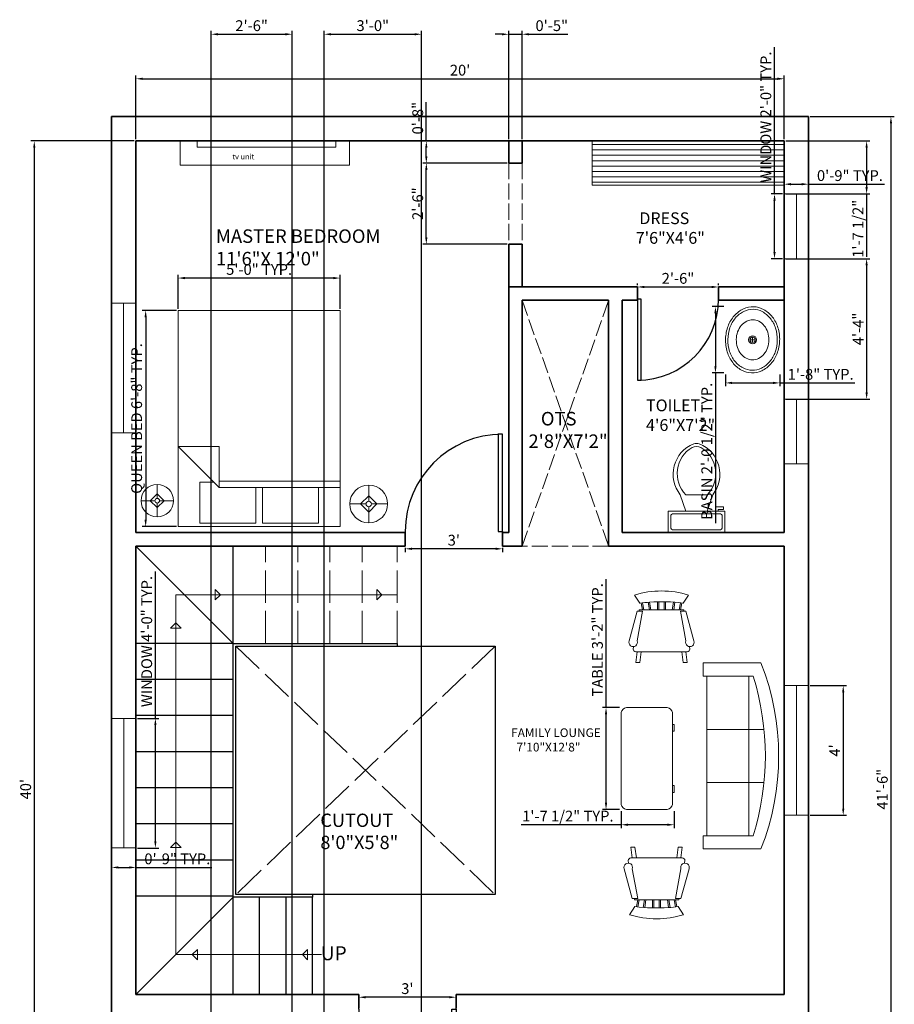
# Model space of a CAD drawing. Units: inches. Extents: x 2170 to 3011, y 1733 to 2338.
# Tile 5 of 5: x 2677 to 3000, y 1974 to 2338. Entities that reach past the tile are written whole.
import ezdxf

# ---------------------------------------------------------------- set-up
doc = ezdxf.new("R2010")
doc.units = ezdxf.units.IN
doc.linetypes.add('ACAD_ISO02W100', pattern=[15, 12, -3])
for name, color, linetype, lineweight in [('A-ANNO-SYMB', 2, 'Continuous', 13), ('A-AREA-IDEN', 4, 'Continuous', 18), ('A-FLOR-CASE', 20, 'Continuous', 20), ('A-FLOR-CASE-PATT', 252, 'Continuous', 13), ('A-FLOR-FIXT', 20, 'Continuous', 18), ('A-FLOR-OPEN', 7, 'Continuous', 25), ('A-FLOR-OPEN-HIDN', 7, 'ACAD_ISO02W100', 13), ('A-FLOR-STRS-OVHD', 150, 'ACAD_ISO02W100', 18), ('A-WALL', 7, 'Continuous', 35), ('A-WALL-OVHD', 7, 'ACAD_ISO02W100', 18), ('dim', 11, 'Continuous', 18), ('door', 6, 'Continuous', 25), ('furnitures', 20, 'Continuous', 18), ('stairs', 150, 'Continuous', 25), ('text', 4, 'Continuous', 18), ('window', 3, 'Continuous', 20)]:
    doc.layers.add(name, color=color, linetype=linetype, lineweight=lineweight)
doc.styles.get("Standard").update_dxf_attribs({"font": 'arial.ttf'})
doc.dimstyles.new('ISO-25', dxfattribs={"dimtxt": 4, "dimasz": 2.5, "dimexe": 1.25, "dimexo": 0.625, "dimtad": 1, "dimlunit": 3, "dimtxsty": 'Standard', "dimcen": 2.5, "dimadec": 0, "dimazin": 0, "dimtfac": 1, "dimtmove": 0, "dimatfit": 3, "dimfxl": 1, "dimarcsym": 0})

# ---------------------------------------------------------------- blocks, each defined once
blk = doc.blocks.new('*U3')
for p, q in [((0, 0), (0, -6)), ((-40, 0), (-40, -6))]:
    blk.add_line(p, q)
blk.add_lwpolyline([(0, 0), (0, 40), (-1.75, 40), (-1.75, 0)], close=True)
blk.add_arc((0, 0), 40, 90, 180)
blk = doc.blocks.new('Toilet - top')
for p, q in [((9.5, -6), (9.5, -2)), ((-10, -8.5), (-8, -8.5)), ((-10, -9.5), (-10, -8.5)), ((-7, -9.5), (-10, -9.5)), ((-8, -8.5), (-8, -8)), ((-7, -8), (-7, -9.5)), ((-4, -8), (-6, -14)), ((4, -8), (6, -14)), ((4, -14), (-4, -14))]:
    blk.add_line(p, q)
blk.add_lwpolyline([(10.5, -8), (10.5, 0), (-10.5, 0), (-10.5, -8)], close=True)
for points in [[(-9.5, -2), (-9.5, -6)], [(8.5, -1), (-8.5, -1)], [(-8.5, -7), (8.5, -7)]]:
    blk.add_lwpolyline(points)
for centre, radius, start, end in [((-8.62, -1.88), 0.884, 81.8699, 188.1301), ((8.62, -1.88), 0.884, 351.8699, 98.1301), ((-8.62, -6.12), 0.884, 171.8699, 278.1301), ((8.62, -6.12), 0.884, 261.8699, 8.1301), ((3.52, -21.58), 12.17, 141.4691, 247.9714), ((4.2, -21.82), 11.33, 136.3677, 238.9468), ((-3.52, -21.58), 12.17, 292.0284, 38.5307), ((-4.2, -21.82), 11.33, 301.053, 43.6321), ((0, -27.88), 4, 245.7318, 294.2682), ((0, -29), 4, 254.8605, 285.1395)]:
    blk.add_arc(centre, radius, start, end)
blk = doc.blocks.new('Bed - Queen')
for p, q in [((0, -80.00003), (0, 0)), ((0, 0), (59.99999, 0)), ((59.99999, 0), (59.99999, -80.00003)), ((7.99999, -1.2), (28.79998, -1.2)), ((7.99999, -14.4), (7.99999, -1.2)), ((28.79998, -1.2), (28.79998, -14.4)), ((31.19999, -1.2), (51.99999, -1.2)), ((31.19999, -14.4), (31.19999, -1.2)), ((51.99999, -1.2), (51.99999, -16.4)), ((0, -14.4), (44.8, -14.4)), ((59.99999, -29.6), (44.8, -14.4)), ((44.8, -14.4), (44.8, -29.6)), ((44.8, -16.8), (0, -16.8)), ((51.99999, -16.4), (46.79936, -16.4)), ((44.8, -29.6), (59.99999, -29.6)), ((59.99999, -80.00003), (0, -80.00003))]:
    blk.add_line(p, q)
blk = doc.blocks.new('Desk - 30 x 60 in.')
for p, q in [((-26.999995, 0), (26.999995, 0)), ((-29.999995, -27), (-29.999995, -3)), ((29.999995, -3), (29.999995, -27)), ((26.999995, -30), (-26.999995, -30)), ((-20.000005, -30), (-20.000005, -31)), ((-20.000005, -31), (-16.000005, -31)), ((-16.000005, -31), (-16.000005, -30)), ((15.999995, -31), (15.999995, -30)), ((19.999995, -31), (15.999995, -31)), ((19.999995, -30), (19.999995, -31))]:
    blk.add_line(p, q)
for centre, start, end in [((-26.499995, -3.5), 98.1301, 171.8699), ((26.499995, -3.5), 8.130102, 81.8699), ((-26.499995, -26.5), 188.1301, 261.8699), ((26.499995, -26.5), 278.1301, 351.8699)]:
    blk.add_arc(centre, 3.535534, start, end)
blk = doc.blocks.new('Sofa - Roundback 7 ft.')
for p, q in [((-12.00002, -32.4421), (-12.00003, -6.5971)), ((11.99997, -32.4421), (11.99998, -6.5971)), ((-36.000027, -34), (-36.000027, -11.4696)), ((35.99998, -34), (35.99998, -11.4696)), ((-35.999844, -13.3819), (35.9998, -13.3819)), ((-36.000027, -32.4421), (35.99998, -32.4421))]:
    blk.add_line(p, q)
for points in [[(-36.000027, -34), (-42.000027, -34), (-42.000027, -8)], [(41.99998, -8), (41.99998, -34), (35.99998, -34)]]:
    blk.add_lwpolyline(points)
for centre, radius, start, end in [((0, -114.25), 114.25, 68.43141, 111.5686), ((-0.00001, -127.1968), 121.1968, 72.72033, 107.2797)]:
    blk.add_arc(centre, radius, start, end)
blk = doc.blocks.new('Lamp - Table')
for p, q in [((0, 7), (0, 1)), ((-1, 0), (-7, 0)), ((0, 3), (-3, 0)), ((-3, 0), (0, -3)), ((3, 0), (0, 3)), ((0, -3), (3, 0)), ((1, 0), (7, 0)), ((0, -1), (0, -7))]:
    blk.add_line(p, q)
for radius in [7, 1]:
    blk.add_circle((0, 0), radius)
blk = doc.blocks.new('Sink - Oval top')
for p, q in [((-1, 0), (1, 0)), ((0, 1), (0, -1))]:
    blk.add_line(p, q)
for points in [[(-12.23, 0.39, 0.117634), (-11.46, -3.36, 0.104469), (-8.88, -6.8, 0.090016), (-5.08, -9.07, 0.08192), (-0.32, -10.02, 0.08192), (4.49, -9.38, 0.090016), (8.42, -7.36, 0.104469), (11.22, -4.09, 0.117634), (12.23, -0.39, 0.117634), (11.46, 3.36, 0.104469), (8.88, 6.8, 0.090016), (5.08, 9.07, 0.08192), (0.32, 10.02, 0.08192), (-4.49, 9.38, 0.090016), (-8.42, 7.36, 0.104469), (-11.22, 4.09, 0.117634)], [(-11.29, 0.16, 0.118622), (-10.52, -3.25, 0.104678), (-8.07, -6.36, 0.089562), (-4.54, -8.37, 0.081185), (-0.13, -9.15, 0.081185), (4.3, -8.49, 0.089562), (7.89, -6.58, 0.104678), (10.42, -3.55, 0.118622), (11.29, -0.16, 0.118622), (10.52, 3.25, 0.104678), (8.07, 6.36, 0.089562), (4.54, 8.37, 0.081185), (0.13, 9.15, 0.081185), (-4.3, 8.49, 0.089562), (-7.89, 6.58, 0.104678), (-10.42, 3.55, 0.118622)], [(-7.42, 0.08, 0.118283), (-6.91, -2.17, 0.104607), (-5.29, -4.21, 0.089718), (-2.97, -5.53, 0.081436), (-0.07, -6.04, 0.081436), (2.84, -5.59, 0.089718), (5.2, -4.33, 0.104607), (6.86, -2.32, 0.118283), (7.42, -0.08, 0.118283), (6.91, 2.17, 0.104607), (5.29, 4.21, 0.089718), (2.97, 5.53, 0.081436), (0.07, 6.04, 0.081436), (-2.84, 5.59, 0.089718), (-5.2, 4.33, 0.104607), (-6.86, 2.32, 0.118283)]]:
    blk.add_lwpolyline(points, format="xyb", close=True)
for radius in [1.5, 1]:
    blk.add_circle((0, 0), radius)
blk = doc.blocks.new('Chair - Rocking')
for p, q in [((-8, -4.5), (-10, -1.5)), ((8, -4.5), (10, -1.5)), ((-8.23428, -6.99939), (-8.3093, -7.47958)), ((-8.23041, -7), (8.23915, -7)), ((-7.5, -4.5), (-7, -7)), ((-6.5, -7), (-7.02225, -4.43)), ((-4.5, -7), (-4.96674, -4.19951)), ((-4, -7), (-4.40532, -4.16272)), ((-1.5, -4.05012), (-1.5, -7)), ((-1, -7), (-1, -4.05012)), ((1, -7), (1, -4.04655)), ((1.5, -4.05012), (1.5, -7)), ((4, -7), (4.40187, -4.18694)), ((4.5, -7), (4.96761, -4.19437)), ((6.5, -7), (7, -4.4057)), ((7.5, -4.5), (7, -7)), ((8.31071, -7.48854), (8.23449, -7.00073)), ((-9, -7.5), (-12, -18.49999)), ((-7, -7.5), (-9, -7.5)), ((-9, -18.49999), (-7, -7.5)), ((7, -7.5), (9, -7.5)), ((9, -18.49999), (7, -7.5)), ((9, -7.5), (12, -18.49999)), ((-10.36644, -20.64523), (-10.5, -21.49999)), ((10.5, -21.49999), (10.3575, -20.58798)), ((-9, -22.49999), (-9.5, -26.49999)), ((0, -22.49999), (-9.5, -22.49999)), ((-8, -26.49999), (-7.5, -22.49999)), ((0, -22.49999), (9.5, -22.49999)), ((8, -26.49999), (7.5, -22.49999)), ((9, -22.49999), (9.5, -26.49999)), ((-9.5, -26.49999), (-8, -26.49999)), ((9.5, -26.49999), (8, -26.49999))]:
    blk.add_line(p, q)
for centre, radius, start, end in [((0, -34.08333), 34.08333, 72.93847, 107.0615), ((0, -68.25004), 64.25, 93.92211, 97.15267), ((0, -68.25004), 64.25, 82.84733, 93.92211), ((-10.5, -18.99999), 1.58114, 161.5651, 18.43495), ((-9.5, -21.49999), 1, 180, 270), ((10.5, -18.99999), 1.58114, 161.5651, 18.43495), ((9.5, -21.49999), 1, 270, 0)]:
    blk.add_arc(centre, radius, start, end)
blk = doc.blocks.new('*D35')
at = {"layer": 'Defpoints', "color": 0, "transparency": 16777216}
for p in [(2959.6, 2316.33), (2719.6, 2293.31), (2959.6, 2293.31)]:
    blk.add_point(p, dxfattribs=at)
at = {"layer": 'dim', "color": 0, "lineweight": -2, "transparency": 16777216}
for p, q in [((2719.6, 2293.93), (2719.6, 2317.58)), ((2722.1, 2316.33), (2957.1, 2316.33)), ((2959.6, 2293.93), (2959.6, 2317.58))]:
    blk.add_line(p, q, dxfattribs=at)
at = {"layer": 'dim', "color": 0, "transparency": 16777216}
for points in [[(2722.1, 2316.74), (2722.1, 2315.91), (2719.6, 2316.33)], [(2957.1, 2316.74), (2957.1, 2315.91), (2959.6, 2316.33)]]:
    blk.add_solid(points, dxfattribs=at)
at = {"layer": 'dim', "color": 0, "transparency": 16777216, "insert": (2839.6, 2318.99), "char_height": 4, "attachment_point": 5}
blk.add_mtext("20'", dxfattribs=at)
blk = doc.blocks.new('*D36')
at = {"layer": 'Defpoints', "color": 0, "transparency": 16777216}
for p in [(2719.6, 2293.31), (2681.96, 1813.31), (2719.6, 1813.31)]:
    blk.add_point(p, dxfattribs=at)
at = {"layer": 'dim', "color": 0, "lineweight": -2, "transparency": 16777216}
for p, q in [((2718.97, 2293.31), (2680.71, 2293.31)), ((2681.96, 2290.81), (2681.96, 1815.81)), ((2718.97, 1813.31), (2680.71, 1813.31))]:
    blk.add_line(p, q, dxfattribs=at)
at = {"layer": 'dim', "color": 0, "transparency": 16777216}
for points in [[(2681.54, 2290.81), (2682.37, 2290.81), (2681.96, 2293.31)], [(2681.54, 1815.81), (2682.37, 1815.81), (2681.96, 1813.31)]]:
    blk.add_solid(points, dxfattribs=at)
at = {"layer": 'dim', "color": 0, "transparency": 16777216, "insert": (2679.29, 2053.31), "char_height": 4, "attachment_point": 5, "rotation": 90}
blk.add_mtext("40'", dxfattribs=at)
blk = doc.blocks.new('*D33')
at = {"layer": 'Defpoints', "color": 0, "transparency": 16777216}
for p in [(2819.27, 2143.31), (2819.27, 2142.31), (2855.27, 2143.31)]:
    blk.add_point(p, dxfattribs=at)
at = {"layer": 'dim', "color": 0, "lineweight": -2, "transparency": 16777216}
for p, q in [((2819.27, 2142.68), (2819.27, 2141.06)), ((2852.77, 2142.31), (2821.77, 2142.31)), ((2855.27, 2142.68), (2855.27, 2141.06))]:
    blk.add_line(p, q, dxfattribs=at)
at = {"layer": 'dim', "color": 0, "transparency": 16777216}
for points in [[(2821.77, 2142.73), (2821.77, 2141.9), (2819.27, 2142.31)], [(2852.77, 2142.73), (2852.77, 2141.9), (2855.27, 2142.31)]]:
    blk.add_solid(points, dxfattribs=at)
at = {"layer": 'dim', "color": 0, "transparency": 16777216, "insert": (2837.27, 2144.98), "char_height": 4, "attachment_point": 5}
blk.add_mtext("3'", dxfattribs=at)
blk = doc.blocks.new('*D34')
at = {"layer": 'Defpoints', "color": 0, "transparency": 16777216}
for p in [(2968.6, 2091.66), (2968.6, 2043.66), (2981.44, 2043.66)]:
    blk.add_point(p, dxfattribs=at)
at = {"layer": 'dim', "color": 0, "lineweight": -2, "transparency": 16777216}
for p, q in [((2969.22, 2091.66), (2982.69, 2091.66)), ((2981.44, 2089.16), (2981.44, 2046.16)), ((2969.22, 2043.66), (2982.69, 2043.66))]:
    blk.add_line(p, q, dxfattribs=at)
at = {"layer": 'dim', "color": 0, "transparency": 16777216}
for points in [[(2981.03, 2089.16), (2981.86, 2089.16), (2981.44, 2091.66)], [(2981.03, 2046.16), (2981.86, 2046.16), (2981.44, 2043.66)]]:
    blk.add_solid(points, dxfattribs=at)
at = {"layer": 'dim', "color": 0, "transparency": 16777216, "insert": (2978.82, 2067.66), "char_height": 4, "attachment_point": 5, "rotation": 90}
blk.add_mtext("4'", dxfattribs=at)
blk = doc.blocks.new('*U37')
for p, q in [((-40, 0), (-40, 6)), ((0, 0), (0, 6))]:
    blk.add_line(p, q)
blk.add_lwpolyline([(0, 0), (0, -40), (-1.75, -40), (-1.75, 0)], close=True)
blk.add_arc((0, 0), 40, 180, 270)
blk = doc.blocks.new('*D41')
at = {"layer": 'Defpoints', "color": 0, "transparency": 16777216}
for p in [(2802.09, 1977.31), (2802.09, 1976.29), (2838.09, 1977.31)]:
    blk.add_point(p, dxfattribs=at)
at = {"layer": 'dim', "color": 0, "lineweight": -2, "transparency": 16777216}
for p, q in [((2802.09, 1976.68), (2802.09, 1975.04)), ((2835.59, 1976.29), (2804.59, 1976.29)), ((2838.09, 1976.68), (2838.09, 1975.04))]:
    blk.add_line(p, q, dxfattribs=at)
at = {"layer": 'dim', "color": 0, "transparency": 16777216}
for points in [[(2804.59, 1976.71), (2804.59, 1975.88), (2802.09, 1976.29)], [(2835.59, 1976.71), (2835.59, 1975.88), (2838.09, 1976.29)]]:
    blk.add_solid(points, dxfattribs=at)
at = {"layer": 'dim', "color": 0, "transparency": 16777216, "insert": (2820.09, 1978.96), "char_height": 4, "attachment_point": 5}
blk.add_mtext("3'", dxfattribs=at)
blk = doc.blocks.new('*D42')
at = {"layer": 'Defpoints', "color": 0, "transparency": 16777216}
for p in [(2905.27, 2239.26), (2935.27, 2239.26), (2935.27, 2239.26)]:
    blk.add_point(p, dxfattribs=at)
at = {"layer": 'dim', "color": 0, "lineweight": -2, "transparency": 16777216}
for p, q in [((2905.27, 2239.88), (2905.27, 2240.51)), ((2907.77, 2239.26), (2932.77, 2239.26)), ((2935.27, 2239.88), (2935.27, 2240.51))]:
    blk.add_line(p, q, dxfattribs=at)
at = {"layer": 'dim', "color": 0, "transparency": 16777216}
for points in [[(2907.77, 2239.67), (2907.77, 2238.84), (2905.27, 2239.26)], [(2932.77, 2239.67), (2932.77, 2238.84), (2935.27, 2239.26)]]:
    blk.add_solid(points, dxfattribs=at)
at = {"layer": 'dim', "color": 0, "transparency": 16777216, "insert": (2920.27, 2241.92), "char_height": 4, "attachment_point": 5}
blk.add_mtext('2\'-6"', dxfattribs=at)
blk = doc.blocks.new('WINDOW-48x9')
blk.add_line((4.5, 48), (4.5, 0))
blk.add_lwpolyline([(0, 48), (9, 48), (9, 0), (0, 0)], close=True)
blk = doc.blocks.new('WINDOW-24x9')
blk.add_line((4.5, 24), (4.5, 0))
blk.add_lwpolyline([(0, 24), (9, 24), (9, 0), (0, 0)], close=True)
blk = doc.blocks.new('STAIR-UP-PATH')
for p, q in [((1.94, 1.94), (1.94, 135.18)), ((1.94, 135.18), (83.94, 135.18)), ((16.56, 133.24), (16.56, 137.12)), ((16.56, 137.12), (18.45, 135.18)), ((16.56, 133.24), (18.45, 135.18)), ((76.31, 133.24), (76.31, 137.12)), ((76.31, 137.12), (78.21, 135.18)), ((76.31, 133.24), (78.21, 135.18)), ((0, 122.86), (1.94, 124.75)), ((3.88, 122.86), (1.94, 124.75)), ((3.88, 122.86), (0, 122.86)), ((0, 41.63), (1.94, 43.52)), ((3.88, 41.63), (0, 41.63)), ((3.88, 41.63), (1.94, 43.52)), ((9.93, 3.88), (8.04, 1.94)), ((9.93, 3.88), (9.93, 0)), ((50.68, 3.88), (48.79, 1.94)), ((50.68, 3.88), (50.68, 0)), ((55.9, 1.94), (1.94, 1.94)), ((9.93, 0), (8.04, 1.94)), ((50.68, 0), (48.79, 1.94))]:
    blk.add_line(p, q)
blk = doc.blocks.new('*D56')
at = {"layer": 'Defpoints', "color": 0, "transparency": 16777216}
for p in [(2937.82, 2231.97), (2934.14, 2207.42), (2937.82, 2207.42)]:
    blk.add_point(p, dxfattribs=at)
at = {"layer": 'dim', "color": 0, "lineweight": -2, "transparency": 16777216}
for p, q in [((2937.2, 2231.97), (2932.89, 2231.97)), ((2934.14, 2229.47), (2934.14, 2209.92)), ((2937.2, 2207.42), (2932.89, 2207.42)), ((2934.14, 2207.42), (2934.14, 2151.82))]:
    blk.add_line(p, q, dxfattribs=at)
at = {"layer": 'dim', "color": 0, "transparency": 16777216}
for points in [[(2933.72, 2229.47), (2934.55, 2229.47), (2934.14, 2231.97)], [(2933.72, 2209.92), (2934.55, 2209.92), (2934.14, 2207.42)]]:
    blk.add_solid(points, dxfattribs=at)
at = {"layer": 'dim', "color": 0, "transparency": 16777216, "insert": (2931.44, 2178.37), "char_height": 4, "attachment_point": 5, "rotation": 90}
blk.add_mtext('BASIN 2\'-0 1/2" TYP.', dxfattribs=at)
blk = doc.blocks.new('*D57')
at = {"layer": 'Defpoints', "color": 0, "transparency": 16777216}
for p in [(2937.82, 2207.42), (2957.96, 2207.42), (2957.96, 2203.73)]:
    blk.add_point(p, dxfattribs=at)
at = {"layer": 'dim', "color": 0, "lineweight": -2, "transparency": 16777216}
for p, q in [((2937.82, 2206.79), (2937.82, 2202.48)), ((2957.96, 2206.79), (2957.96, 2202.48)), ((2940.32, 2203.73), (2955.46, 2203.73)), ((2957.96, 2203.73), (2985.71, 2203.73))]:
    blk.add_line(p, q, dxfattribs=at)
at = {"layer": 'dim', "color": 0, "transparency": 16777216}
for points in [[(2940.32, 2204.15), (2940.32, 2203.32), (2937.82, 2203.73)], [(2955.46, 2204.15), (2955.46, 2203.32), (2957.96, 2203.73)]]:
    blk.add_solid(points, dxfattribs=at)
at = {"layer": 'dim', "color": 0, "transparency": 16777216, "insert": (2973.08, 2206.4), "char_height": 4, "attachment_point": 5}
blk.add_mtext('1\'-8" TYP.', dxfattribs=at)
blk = doc.blocks.new('*D60')
at = {"layer": 'Defpoints', "color": 0, "transparency": 16777216}
for p in [(2735.2, 2230.55), (2723.2, 2150.55), (2735.2, 2150.55)]:
    blk.add_point(p, dxfattribs=at)
at = {"layer": 'dim', "color": 0, "lineweight": -2, "transparency": 16777216}
for p, q in [((2734.57, 2230.55), (2721.95, 2230.55)), ((2723.2, 2228.05), (2723.2, 2153.05)), ((2734.57, 2150.55), (2721.95, 2150.55))]:
    blk.add_line(p, q, dxfattribs=at)
at = {"layer": 'dim', "color": 0, "transparency": 16777216}
for points in [[(2722.78, 2228.05), (2723.61, 2228.05), (2723.2, 2230.55)], [(2722.78, 2153.05), (2723.61, 2153.05), (2723.2, 2150.55)]]:
    blk.add_solid(points, dxfattribs=at)
at = {"layer": 'dim', "color": 0, "transparency": 16777216, "insert": (2720.38, 2190.55), "char_height": 4, "attachment_point": 5, "rotation": 90}
blk.add_mtext('QUEEN BED 6\'-8" TYP.', dxfattribs=at)
blk = doc.blocks.new('*D61')
at = {"layer": 'Defpoints', "color": 0, "transparency": 16777216}
for p in [(2735.2, 2242.55), (2735.2, 2230.55), (2795.2, 2230.55)]:
    blk.add_point(p, dxfattribs=at)
at = {"layer": 'dim', "color": 0, "lineweight": -2, "transparency": 16777216}
for p, q in [((2735.2, 2231.17), (2735.2, 2243.8)), ((2792.7, 2242.55), (2737.7, 2242.55)), ((2795.2, 2231.17), (2795.2, 2243.8))]:
    blk.add_line(p, q, dxfattribs=at)
at = {"layer": 'dim', "color": 0, "transparency": 16777216}
for points in [[(2737.7, 2242.96), (2737.7, 2242.13), (2735.2, 2242.55)], [(2792.7, 2242.96), (2792.7, 2242.13), (2795.2, 2242.55)]]:
    blk.add_solid(points, dxfattribs=at)
at = {"layer": 'dim', "color": 0, "transparency": 16777216, "insert": (2765.2, 2245.22), "char_height": 4, "attachment_point": 5}
blk.add_mtext('5\'-0" TYP.', dxfattribs=at)
blk = doc.blocks.new('*D62')
at = {"layer": 'Defpoints', "color": 0, "transparency": 16777216}
for p in [(2893.63, 2083.58), (2899.29, 2083.58), (2899.29, 2045.81)]:
    blk.add_point(p, dxfattribs=at)
at = {"layer": 'dim', "color": 0, "lineweight": -2, "transparency": 16777216}
for p, q in [((2893.63, 2083.58), (2893.63, 2131.07)), ((2898.67, 2083.58), (2892.38, 2083.58)), ((2893.63, 2048.31), (2893.63, 2081.08)), ((2898.67, 2045.81), (2892.38, 2045.81))]:
    blk.add_line(p, q, dxfattribs=at)
at = {"layer": 'dim', "color": 0, "transparency": 16777216}
for points in [[(2893.21, 2081.08), (2894.04, 2081.08), (2893.63, 2083.58)], [(2893.21, 2048.31), (2894.04, 2048.31), (2893.63, 2045.81)]]:
    blk.add_solid(points, dxfattribs=at)
at = {"layer": 'dim', "color": 0, "transparency": 16777216, "insert": (2890.96, 2108.58), "char_height": 4, "attachment_point": 5, "rotation": 90}
blk.add_mtext('TABLE 3\'-2" TYP.', dxfattribs=at)
blk = doc.blocks.new('*D63')
at = {"layer": 'Defpoints', "color": 0, "transparency": 16777216}
for p in [(2899.29, 2045.81), (2918.8, 2045.81), (2899.29, 2040.15)]:
    blk.add_point(p, dxfattribs=at)
at = {"layer": 'dim', "color": 0, "lineweight": -2, "transparency": 16777216}
for p, q in [((2899.29, 2045.19), (2899.29, 2038.9)), ((2918.8, 2045.19), (2918.8, 2038.9)), ((2899.29, 2040.15), (2862.22, 2040.15)), ((2916.3, 2040.15), (2901.79, 2040.15))]:
    blk.add_line(p, q, dxfattribs=at)
at = {"layer": 'dim', "color": 0, "transparency": 16777216}
for points in [[(2901.79, 2040.57), (2901.79, 2039.73), (2899.29, 2040.15)], [(2916.3, 2040.57), (2916.3, 2039.73), (2918.8, 2040.15)]]:
    blk.add_solid(points, dxfattribs=at)
at = {"layer": 'dim', "color": 0, "transparency": 16777216, "insert": (2879.5, 2042.84), "char_height": 4, "attachment_point": 5}
blk.add_mtext('1\'-7 1/2" TYP.', dxfattribs=at)
blk = doc.blocks.new('*D78')
at = {"layer": 'Defpoints', "color": 0, "transparency": 16777216}
for p in [(2719.6, 2079.54), (2726.8, 2079.54), (2719.6, 2031.54)]:
    blk.add_point(p, dxfattribs=at)
at = {"layer": 'dim', "color": 0, "lineweight": -2, "transparency": 16777216}
for p, q in [((2726.8, 2079.54), (2726.8, 2133.91)), ((2720.22, 2079.54), (2728.05, 2079.54)), ((2726.8, 2034.04), (2726.8, 2077.04)), ((2720.22, 2031.54), (2728.05, 2031.54))]:
    blk.add_line(p, q, dxfattribs=at)
at = {"layer": 'dim', "color": 0, "transparency": 16777216}
for points in [[(2726.38, 2077.04), (2727.22, 2077.04), (2726.8, 2079.54)], [(2726.38, 2034.04), (2727.22, 2034.04), (2726.8, 2031.54)]]:
    blk.add_solid(points, dxfattribs=at)
at = {"layer": 'dim', "color": 0, "transparency": 16777216, "insert": (2724.11, 2107.98), "char_height": 4, "attachment_point": 5, "rotation": 90}
blk.add_mtext('WINDOW 4\'-0" TYP.', dxfattribs=at)
blk = doc.blocks.new('*D79')
at = {"layer": 'Defpoints', "color": 0, "transparency": 16777216}
for p in [(2710.6, 2031.54), (2719.6, 2031.54), (2719.6, 2024.34)]:
    blk.add_point(p, dxfattribs=at)
at = {"layer": 'dim', "color": 0, "lineweight": -2, "transparency": 16777216}
for p, q in [((2710.6, 2030.92), (2710.6, 2023.09)), ((2719.6, 2030.92), (2719.6, 2023.09)), ((2713.1, 2024.34), (2717.1, 2024.34)), ((2719.6, 2024.34), (2747.73, 2024.34))]:
    blk.add_line(p, q, dxfattribs=at)
at = {"layer": 'dim', "color": 0, "transparency": 16777216}
for points in [[(2713.1, 2024.76), (2713.1, 2023.93), (2710.6, 2024.34)], [(2717.1, 2024.76), (2717.1, 2023.93), (2719.6, 2024.34)]]:
    blk.add_solid(points, dxfattribs=at)
at = {"layer": 'dim', "color": 0, "transparency": 16777216, "insert": (2734.92, 2027.01), "char_height": 4, "attachment_point": 5}
blk.add_mtext('0\'-9" TYP.', dxfattribs=at)
blk = doc.blocks.new('*D80')
at = {"layer": 'Defpoints', "color": 0, "transparency": 16777216}
for p in [(2956, 2273.7), (2959.6, 2273.7), (2959.6, 2249.7)]:
    blk.add_point(p, dxfattribs=at)
at = {"layer": 'dim', "color": 0, "lineweight": -2, "transparency": 16777216}
for p, q in [((2956, 2273.7), (2956, 2328.07)), ((2958.97, 2273.7), (2954.75, 2273.7)), ((2956, 2252.2), (2956, 2271.2)), ((2958.97, 2249.7), (2954.75, 2249.7))]:
    blk.add_line(p, q, dxfattribs=at)
at = {"layer": 'dim', "color": 0, "transparency": 16777216}
for points in [[(2955.58, 2271.2), (2956.42, 2271.2), (2956, 2273.7)], [(2955.58, 2252.2), (2956.42, 2252.2), (2956, 2249.7)]]:
    blk.add_solid(points, dxfattribs=at)
at = {"layer": 'dim', "color": 0, "transparency": 16777216, "insert": (2953.31, 2302.13), "char_height": 4, "attachment_point": 5, "rotation": 90}
blk.add_mtext('WINDOW 2\'-0" TYP.', dxfattribs=at)
blk = doc.blocks.new('*D81')
at = {"layer": 'Defpoints', "color": 0, "transparency": 16777216}
for p in [(2968.6, 2277.3), (2959.6, 2273.7), (2968.6, 2273.7)]:
    blk.add_point(p, dxfattribs=at)
at = {"layer": 'dim', "color": 0, "lineweight": -2, "transparency": 16777216}
for p, q in [((2959.6, 2274.32), (2959.6, 2278.55)), ((2968.6, 2274.32), (2968.6, 2278.55)), ((2962.1, 2277.3), (2966.1, 2277.3)), ((2968.6, 2277.3), (2996.73, 2277.3))]:
    blk.add_line(p, q, dxfattribs=at)
at = {"layer": 'dim', "color": 0, "transparency": 16777216}
for points in [[(2962.1, 2277.72), (2962.1, 2276.88), (2959.6, 2277.3)], [(2966.1, 2277.72), (2966.1, 2276.88), (2968.6, 2277.3)]]:
    blk.add_solid(points, dxfattribs=at)
at = {"layer": 'dim', "color": 0, "transparency": 16777216, "insert": (2983.92, 2279.97), "char_height": 4, "attachment_point": 5}
blk.add_mtext('0\'-9" TYP.', dxfattribs=at)
blk = doc.blocks.new('*D82')
at = {"layer": 'Defpoints', "color": 0, "transparency": 16777216}
for p in [(2862.6, 2332.81), (2857.6, 2293.31), (2862.6, 2293.31)]:
    blk.add_point(p, dxfattribs=at)
at = {"layer": 'dim', "color": 0, "lineweight": -2, "transparency": 16777216}
for p, q in [((2857.6, 2293.93), (2857.6, 2334.06)), ((2862.6, 2293.93), (2862.6, 2334.06)), ((2855.1, 2332.81), (2852.6, 2332.81)), ((2857.6, 2332.81), (2862.6, 2332.81)), ((2865.1, 2332.81), (2879.48, 2332.81))]:
    blk.add_line(p, q, dxfattribs=at)
at = {"layer": 'dim', "color": 0, "transparency": 16777216}
for points in [[(2855.1, 2333.22), (2855.1, 2332.39), (2857.6, 2332.81)], [(2865.1, 2333.22), (2865.1, 2332.39), (2862.6, 2332.81)]]:
    blk.add_solid(points, dxfattribs=at)
at = {"layer": 'dim', "color": 0, "transparency": 16777216, "insert": (2873.54, 2335.47), "char_height": 4, "attachment_point": 5}
blk.add_mtext('0\'-5"', dxfattribs=at)
blk = doc.blocks.new('*D92')
at = {"layer": 'Defpoints', "color": 0, "transparency": 16777216}
for p in [(2959.6, 2293.31), (2959.6, 2273.7), (2990.1, 2273.7)]:
    blk.add_point(p, dxfattribs=at)
at = {"layer": 'dim', "color": 0, "lineweight": -2, "transparency": 16777216}
for p, q in [((2960.22, 2293.31), (2991.35, 2293.31)), ((2990.1, 2290.81), (2990.1, 2276.2)), ((2960.22, 2273.7), (2991.35, 2273.7)), ((2990.1, 2273.7), (2990.1, 2250.37))]:
    blk.add_line(p, q, dxfattribs=at)
at = {"layer": 'dim', "color": 0, "transparency": 16777216}
for points in [[(2989.68, 2290.81), (2990.52, 2290.81), (2990.1, 2293.31)], [(2989.68, 2276.2), (2990.52, 2276.2), (2990.1, 2273.7)]]:
    blk.add_solid(points, dxfattribs=at)
at = {"layer": 'dim', "color": 0, "transparency": 16777216, "insert": (2987.41, 2260.79), "char_height": 4, "attachment_point": 5, "rotation": 90}
blk.add_mtext('1\'-7 1/2"', dxfattribs=at)
blk = doc.blocks.new('*D93')
at = {"layer": 'Defpoints', "color": 0, "transparency": 16777216}
for p in [(2959.6, 2249.7), (2959.6, 2197.73), (2990.1, 2197.73)]:
    blk.add_point(p, dxfattribs=at)
at = {"layer": 'dim', "color": 0, "lineweight": -2, "transparency": 16777216}
for p, q in [((2960.22, 2249.7), (2991.35, 2249.7)), ((2990.1, 2247.2), (2990.1, 2200.23)), ((2960.22, 2197.73), (2991.35, 2197.73))]:
    blk.add_line(p, q, dxfattribs=at)
at = {"layer": 'dim', "color": 0, "transparency": 16777216}
for points in [[(2989.68, 2247.2), (2990.52, 2247.2), (2990.1, 2249.7)], [(2989.68, 2200.23), (2990.52, 2200.23), (2990.1, 2197.73)]]:
    blk.add_solid(points, dxfattribs=at)
at = {"layer": 'dim', "color": 0, "transparency": 16777216, "insert": (2987.47, 2223.72), "char_height": 4, "attachment_point": 5, "rotation": 90}
blk.add_mtext('4\'-4"', dxfattribs=at)
blk = doc.blocks.new('*D97')
at = {"layer": 'Defpoints', "color": 0, "transparency": 16777216}
for p in [(2825.28, 2332.81), (2789.28, 1855.31), (2825.28, 1855.31)]:
    blk.add_point(p, dxfattribs=at)
at = {"layer": 'dim', "color": 0, "lineweight": -2, "transparency": 16777216}
for p, q in [((2789.28, 1855.93), (2789.28, 2334.06)), ((2825.28, 1855.93), (2825.28, 2334.06)), ((2791.78, 2332.81), (2822.78, 2332.81))]:
    blk.add_line(p, q, dxfattribs=at)
at = {"layer": 'dim', "color": 0, "transparency": 16777216}
for points in [[(2791.78, 2333.22), (2791.78, 2332.39), (2789.28, 2332.81)], [(2822.78, 2333.22), (2822.78, 2332.39), (2825.28, 2332.81)]]:
    blk.add_solid(points, dxfattribs=at)
at = {"layer": 'dim', "color": 0, "transparency": 16777216, "insert": (2807.28, 2335.48), "char_height": 4, "attachment_point": 5}
blk.add_mtext('3\'-0"', dxfattribs=at)
blk = doc.blocks.new('*D98')
at = {"layer": 'Defpoints', "color": 0, "transparency": 16777216}
for p in [(2777.42, 2332.81), (2747.42, 1903.31), (2777.42, 1903.81)]:
    blk.add_point(p, dxfattribs=at)
at = {"layer": 'dim', "color": 0, "lineweight": -2, "transparency": 16777216}
for p, q in [((2747.42, 1903.93), (2747.42, 2334.06)), ((2777.42, 1904.43), (2777.42, 2334.06)), ((2749.92, 2332.81), (2774.92, 2332.81))]:
    blk.add_line(p, q, dxfattribs=at)
at = {"layer": 'dim', "color": 0, "transparency": 16777216}
for points in [[(2749.92, 2333.22), (2749.92, 2332.39), (2747.42, 2332.81)], [(2774.92, 2333.22), (2774.92, 2332.39), (2777.42, 2332.81)]]:
    blk.add_solid(points, dxfattribs=at)
at = {"layer": 'dim', "color": 0, "transparency": 16777216, "insert": (2762.42, 2335.47), "char_height": 4, "attachment_point": 5}
blk.add_mtext('2\'-6"', dxfattribs=at)
blk = doc.blocks.new('*D101')
at = {"layer": 'Defpoints', "color": 0, "transparency": 16777216}
for p in [(2968.6, 2302.31), (2968.6, 1804.31), (2999.1, 1804.31)]:
    blk.add_point(p, dxfattribs=at)
at = {"layer": 'dim', "color": 0, "lineweight": -2, "transparency": 16777216}
for p, q in [((2969.22, 2302.31), (3000.35, 2302.31)), ((2999.1, 2299.81), (2999.1, 1806.81)), ((2969.22, 1804.31), (3000.35, 1804.31))]:
    blk.add_line(p, q, dxfattribs=at)
at = {"layer": 'dim', "color": 0, "transparency": 16777216}
for points in [[(2998.68, 2299.81), (2999.52, 2299.81), (2999.1, 2302.31)], [(2998.68, 1806.81), (2999.52, 1806.81), (2999.1, 1804.31)]]:
    blk.add_solid(points, dxfattribs=at)
at = {"layer": 'dim', "color": 0, "transparency": 16777216, "insert": (2996.43, 2053.31), "char_height": 4, "attachment_point": 5, "rotation": 90}
blk.add_mtext('41\'-6"', dxfattribs=at)
blk = doc.blocks.new('*D103')
at = {"layer": 'Defpoints', "color": 0, "transparency": 16777216}
for p in [(2827.1, 2285.1), (2857.6, 2285.1), (2857.6, 2255.1)]:
    blk.add_point(p, dxfattribs=at)
at = {"layer": 'dim', "color": 0, "lineweight": -2, "transparency": 16777216}
for p, q in [((2856.97, 2285.1), (2825.85, 2285.1)), ((2827.1, 2257.6), (2827.1, 2282.6)), ((2856.97, 2255.1), (2825.85, 2255.1))]:
    blk.add_line(p, q, dxfattribs=at)
at = {"layer": 'dim', "color": 0, "transparency": 16777216}
for points in [[(2826.68, 2282.6), (2827.52, 2282.6), (2827.1, 2285.1)], [(2826.68, 2257.6), (2827.52, 2257.6), (2827.1, 2255.1)]]:
    blk.add_solid(points, dxfattribs=at)
at = {"layer": 'dim', "color": 0, "transparency": 16777216, "insert": (2824.43, 2270.1), "char_height": 4, "attachment_point": 5, "rotation": 90}
blk.add_mtext('2\'-6"', dxfattribs=at)
blk = doc.blocks.new('*D104')
at = {"layer": 'Defpoints', "color": 0, "transparency": 16777216}
for p in [(2827.1, 2293.31), (2857.6, 2293.31), (2857.6, 2285.1)]:
    blk.add_point(p, dxfattribs=at)
at = {"layer": 'dim', "color": 0, "lineweight": -2, "transparency": 16777216}
for p, q in [((2827.1, 2293.31), (2827.1, 2307.69)), ((2856.97, 2293.31), (2825.85, 2293.31)), ((2827.1, 2287.6), (2827.1, 2290.81)), ((2856.97, 2285.1), (2825.85, 2285.1))]:
    blk.add_line(p, q, dxfattribs=at)
at = {"layer": 'dim', "color": 0, "transparency": 16777216}
for points in [[(2826.68, 2290.81), (2827.52, 2290.81), (2827.1, 2293.31)], [(2826.68, 2287.6), (2827.52, 2287.6), (2827.1, 2285.1)]]:
    blk.add_solid(points, dxfattribs=at)
at = {"layer": 'dim', "color": 0, "transparency": 16777216, "insert": (2824.43, 2301.75), "char_height": 4, "attachment_point": 5, "rotation": 90}
blk.add_mtext('0\'-8"', dxfattribs=at)

msp = doc.modelspace()

# ---------------------------------------------------------------- hatches: boundary and pattern name
at = {"layer": 'A-FLOR-CASE-PATT'}
h = msp.add_hatch(dxfattribs=at)
h.set_pattern_fill('ANSI31', color=256, scale=0.629921, angle=-45, style=0)
h.paths.add_polyline_path([(2888.497, 2293.306), (2959.6, 2293.306), (2959.6, 2276.892), (2888.497, 2276.892)])

# ---------------------------------------------------------------- linework, layer by layer
at = {"layer": 'A-FLOR-CASE'}
for p, q in [((2736.017, 2293.306), (2736.017, 2284.394)), ((2742.288, 2293.306), (2742.288, 2290.971)), ((2793.657, 2290.971), (2793.657, 2293.306)), ((2798.626, 2284.394), (2798.626, 2293.306)), ((2888.497, 2293.306), (2959.6, 2293.306)), ((2888.497, 2276.892), (2888.497, 2293.306)), ((2959.6, 2293.306), (2959.6, 2276.892)), ((2742.288, 2290.971), (2793.657, 2290.971)), ((2736.017, 2284.394), (2798.626, 2284.394)), ((2959.6, 2276.892), (2888.497, 2276.892))]:
    msp.add_line(p, q, dxfattribs=at)
at = {"layer": 'A-FLOR-OPEN'}
msp.add_lwpolyline([(2756.6, 2106.306), (2852.6, 2106.306), (2852.6, 2014.306), (2756.6, 2014.306)], close=True, dxfattribs=at)
at = {"layer": 'A-FLOR-OPEN-HIDN', "ltscale": 0.5}
for p, q in [((2862.6, 2234.306), (2894.6, 2143.306)), ((2862.6, 2143.306), (2894.6, 2234.306)), ((2894.6, 2143.306), (2862.6, 2143.306))]:
    msp.add_line(p, q, dxfattribs=at)
at = {"layer": 'A-FLOR-OPEN-HIDN'}
for p, q in [((2756.6, 2106.306), (2852.6, 2014.306)), ((2852.6, 2106.306), (2756.6, 2014.306))]:
    msp.add_line(p, q, dxfattribs=at)
at = {"layer": 'A-FLOR-STRS-OVHD'}
for p, q in [((2767.535, 2107.306), (2767.535, 2143.306)), ((2779.47, 2107.306), (2779.47, 2143.306)), ((2791.405, 2107.306), (2791.405, 2143.306)), ((2803.34, 2107.306), (2803.34, 2143.306)), ((2816.352, 2107.306), (2816.352, 2143.306))]:
    msp.add_line(p, q, dxfattribs=at)
at = {"layer": 'A-WALL'}
for p, q in [((2710.6, 1804.306), (2710.6, 2302.306)), ((2710.6, 2302.306), (2968.6, 2302.306)), ((2968.6, 1804.306), (2968.6, 2302.306)), ((2719.6, 2148.306), (2719.6, 2293.306)), ((2719.6, 2293.306), (2959.6, 2293.306)), ((2857.6, 2285.102), (2857.6, 2293.306)), ((2862.6, 2285.102), (2862.6, 2293.306)), ((2959.6, 2148.306), (2959.6, 2293.306)), ((2862.6, 2285.102), (2857.6, 2285.102)), ((2857.6, 2148.306), (2857.6, 2255.102)), ((2862.6, 2255.102), (2857.6, 2255.102)), ((2862.6, 2239.306), (2862.6, 2255.102)), ((2857.6, 2239.306), (2862.6, 2239.306)), ((2862.6, 2239.306), (2905.267, 2239.257)), ((2935.267, 2239.257), (2959.6, 2239.257)), ((2862.6, 2143.306), (2862.6, 2234.306)), ((2862.6, 2234.306), (2894.6, 2234.306)), ((2894.6, 2234.306), (2862.6, 2234.306)), ((2894.6, 2183.933), (2894.6, 2234.306)), ((2899.6, 2183.933), (2899.6, 2234.306)), ((2899.6, 2234.306), (2905.267, 2234.306)), ((2935.267, 2234.306), (2959.6, 2234.306)), ((2894.6, 2143.306), (2894.6, 2194.652)), ((2899.6, 2148.306), (2899.6, 2194.652)), ((2719.6, 2148.306), (2819.271, 2148.306)), ((2855.271, 2148.306), (2857.6, 2148.306)), ((2899.6, 2148.306), (2959.6, 2148.306)), ((2719.6, 1977.306), (2719.6, 2143.306)), ((2719.6, 2143.306), (2819.271, 2143.306)), ((2855.271, 2143.306), (2862.6, 2143.306)), ((2894.6, 2143.306), (2959.6, 2143.306)), ((2959.6, 1977.306), (2959.6, 2143.306)), ((2719.6, 1977.306), (2784.944, 1977.306)), ((2784.944, 1977.306), (2802.086, 1977.306)), ((2838.086, 1977.306), (2959.6, 1977.306))]:
    msp.add_line(p, q, dxfattribs=at)
for points in [[(2905.267, 2234.257), (2905.267, 2239.257)], [(2935.267, 2239.257), (2935.267, 2234.257)], [(2819.271, 2143.306), (2819.271, 2148.306)], [(2855.271, 2148.306), (2855.271, 2143.306)], [(2802.086, 1972.306), (2802.086, 1977.306)], [(2838.086, 1977.306), (2838.086, 1972.306)]]:
    msp.add_lwpolyline(points, dxfattribs=at)
at = {"layer": 'A-WALL-OVHD', "ltscale": 0.5}
for p, q in [((2857.6, 2285.102), (2857.6, 2255.102)), ((2862.6, 2285.102), (2862.6, 2255.102))]:
    msp.add_line(p, q, dxfattribs=at)
at = {"layer": 'door'}
for points in [[(2819.271, 2143.306), (2819.271, 2148.306)], [(2855.271, 2148.306), (2855.271, 2143.306)]]:
    msp.add_lwpolyline(points, dxfattribs=at)
at = {"layer": 'stairs'}
for p, q in [((2755.6, 2107.306), (2719.6, 2143.306)), ((2755.6, 2107.306), (2755.6, 2143.306)), ((2755.6, 2107.306), (2719.6, 2107.306)), ((2755.6, 2013.306), (2755.6, 2107.306)), ((2755.6, 2107.306), (2791.942, 2107.306)), ((2791.942, 2107.306), (2816.352, 2107.306)), ((2816.352, 2107.306), (2816.352, 2106.306)), ((2756.6, 2014.306), (2756.6, 2106.306)), ((2756.6, 2106.306), (2791.942, 2106.306)), ((2791.942, 2106.306), (2816.352, 2106.306)), ((2755.6, 2093.938), (2719.6, 2093.938)), ((2755.6, 2080.57), (2719.6, 2080.57)), ((2755.6, 2067.202), (2719.6, 2067.202)), ((2755.6, 2053.834), (2719.6, 2053.834)), ((2755.6, 2040.466), (2719.6, 2040.466)), ((2755.6, 2027.098), (2719.6, 2027.098)), ((2755.6, 2013.73), (2719.6, 2013.73)), ((2755.579, 2013.306), (2719.6, 1977.306)), ((2755.579, 1977.306), (2755.579, 2013.306)), ((2784.944, 2013.306), (2755.6, 2013.306)), ((2784.944, 2014.306), (2756.6, 2014.306)), ((2765.368, 1977.306), (2765.368, 2013.306)), ((2775.156, 1977.306), (2775.156, 2013.306)), ((2784.944, 2014.306), (2784.944, 2013.306)), ((2784.944, 1977.306), (2784.944, 2013.306))]:
    msp.add_line(p, q, dxfattribs=at)

# ---------------------------------------------------------------- block references
at = {"layer": 'A-ANNO-SYMB'}
msp.add_blockref('STAIR-UP-PATH', (2732.415, 1990.129), dxfattribs=at)
at = {"layer": 'A-FLOR-FIXT'}
for name, p, rotation in [('Sink - Oval top', (2947.889, 2219.692), 270), ('Toilet - top', (2927.119, 2148.306), 180)]:
    msp.add_blockref(name, p, dxfattribs=dict(at, rotation=rotation))
at = {"layer": 'door', "xscale": 0.75, "yscale": 0.75, "zscale": 0.75, "rotation": 180}
msp.add_blockref('*U3', (2905.267, 2234.757), dxfattribs=at)
at = {"layer": 'door', "xscale": 0.9, "yscale": 0.9, "zscale": 0.9}
for name, p in [('*U3', (2855.271, 2148.706)), ('*U37', (2838.086, 1971.906))]:
    msp.add_blockref(name, p, dxfattribs=at)
at = {"layer": 'furnitures', "rotation": 180}
for name, p in [('Bed - Queen', (2795.198, 2150.548)), ('Chair - Rocking', (2912.351, 2005.354))]:
    msp.add_blockref(name, p, dxfattribs=at)
at = {"layer": 'furnitures', "xscale": 0.8585674405306916, "yscale": 0.8585674405306916, "zscale": 0.8585674405306916}
msp.add_blockref('Lamp - Table', (2727.488, 2160.125), dxfattribs=at)
at = {"layer": 'furnitures'}
for name, p in [('Lamp - Table', (2805.783, 2158.909)), ('Chair - Rocking', (2914.168, 2126.708))]:
    msp.add_blockref(name, p, dxfattribs=at)
for name, p, xscale, yscale, zscale, rotation in [('Sofa - Roundback 7 ft.', (2957.53, 2065.628), 0.820140253862633, 0.820140253862633, 0.820140253862633, 270), ('Desk - 30 x 60 in.', (2899.292, 2064.698), 0.6294377551275093, 0.6294377551275093, 0.6294377551275093, 90)]:
    msp.add_blockref(name, p, dxfattribs=dict(at, xscale=xscale, yscale=yscale, zscale=zscale, rotation=rotation))
at = {"layer": 'window'}
for name, p in [('WINDOW-24x9', (2959.6, 2249.699)), ('WINDOW-48x9', (2710.515, 2185.278)), ('WINDOW-24x9', (2959.6, 2173.732)), ('WINDOW-48x9', (2959.6, 2043.656)), ('WINDOW-48x9', (2710.6, 2031.545))]:
    msp.add_blockref(name, p, dxfattribs=at)

# ---------------------------------------------------------------- texts
at = {"layer": 'A-AREA-IDEN', "attachment_point": 1}
for s, width, gutter_width, insert, char_height in [(' DRESS\\P7\'6"X4\'6"', 43.24627, 10.92, (2904.621, 2266.877), 4.3678), ('MASTER BEDROOM\\P11\'6"X 12\'0"', 81.99853, 12.5, (2749.224, 2260.567), 5), ('TOILET\\P4\'6"X7\'2"', 43.24627, 10.92, (2908.434, 2197.594), 4.3678), ('   OTS\\P2\'8"X7\'2"', 49.50568, 12.5, (2864.91, 2192.985), 5), ('FAMILY LOUNGE\\P  7\'10"X12\'8"', 42.80713, 8.019, (2858.522, 2075.836), 3.20762), ('CUTOUT\\P8\'0"X5\'8"', 48.71482, 12.3, (2787.864, 2044.268), 4.9201)]:
    msp.add_mtext_dynamic_manual_height_columns(s, width=width, gutter_width=gutter_width, heights=[0], dxfattribs=dict(at, insert=insert, char_height=char_height))
at = {"layer": 'text'}
msp.add_text('UP', height=5.1744, dxfattribs=at).set_placement((2788.055, 1989.989))
at = {"layer": 'text', "insert": (2755.273, 2288.488), "char_height": 2, "attachment_point": 1}
msp.add_mtext_dynamic_manual_height_columns('{\\fArial|b1|i1|c0|p34;tv unit}', width=48.71482, gutter_width=12.3, heights=[0], dxfattribs=at)

# ---------------------------------------------------------------- dimensions: what is measured, and where the dimension line sits
at = {"layer": 'dim'}
for base, p1, p2, override, picture, middle in [((2777.416, 2332.806), (2747.42, 1903.306), (2777.416, 1903.806), {"dimdec": 1, "dimlfac": 1, "dimrnd": 0, "dimzin": 1, "dimdsep": 46, "dimlunit": 4, "dimfrac": 2}, '*D98', (2762.418, 2335.474)), ((2825.28, 2332.806), (2789.28, 1855.306), (2825.28, 1855.306), {"dimdec": 1, "dimlfac": 1, "dimrnd": 0, "dimzin": 1, "dimdsep": 46, "dimlunit": 4, "dimfrac": 2}, '*D97', (2807.28, 2335.475)), ((2862.6, 2332.806), (2857.6, 2293.306), (2862.6, 2293.306), {"dimdec": 1, "dimlfac": 1, "dimrnd": 0, "dimzin": 1, "dimdsep": 46, "dimlunit": 4, "dimfrac": 2}, '*D82', (2873.541, 2335.474)), ((2959.6, 2316.325), (2719.6, 2293.306), (2959.6, 2293.306), {"dimclrd": 0, "dimclre": 0, "dimclrt": 0}, '*D35', (2839.6, 2318.992)), ((2935.267, 2239.257), (2905.267, 2239.257), (2935.267, 2239.257), {"dimclrd": 0, "dimclre": 0, "dimclrt": 0}, '*D42', (2920.267, 2241.924)), ((2819.271, 2142.315), (2855.271, 2143.306), (2819.271, 2143.306), {"dimclrd": 0, "dimclre": 0, "dimclrt": 0}, '*D33', (2837.271, 2144.984)), ((2802.086, 1976.293), (2838.086, 1977.306), (2802.086, 1977.306), {"dimclrd": 0, "dimclre": 0, "dimclrt": 0}, '*D41', (2820.086, 1978.962))]:
    dim = msp.add_linear_dim(base=base, p1=p1, p2=p2, dimstyle='ISO-25', override=override, dxfattribs=at)
    dim.commit()
    dim.dimension.update_dxf_attribs({"geometry": picture, "text_midpoint": middle})
for base, p1, p2, angle, text, picture, middle in [((2956, 2273.699), (2959.6, 2249.699), (2959.6, 2273.699), 90, 'WINDOW <> TYP.', '*D80', (2953.305, 2302.132)), ((2735.198, 2242.548), (2795.198, 2230.548), (2735.198, 2230.548), 180, '<> TYP.', '*D61', (2765.198, 2245.215)), ((2934.138, 2207.416), (2937.82, 2231.967), (2937.82, 2207.416), 270, 'BASIN <> TYP.', '*D56', (2931.445, 2178.368)), ((2723.198, 2150.548), (2735.198, 2230.548), (2735.198, 2150.548), 270, 'QUEEN BED <> TYP.', '*D60', (2720.382, 2190.548)), ((2726.8, 2079.545), (2719.6, 2031.545), (2719.6, 2079.545), 90, 'WINDOW <> TYP.', '*D78', (2724.105, 2107.978)), ((2893.627, 2083.581), (2899.292, 2045.815), (2899.292, 2083.581), 90, 'TABLE <> TYP.', '*D62', (2890.959, 2108.575)), ((2899.292, 2040.15), (2918.805, 2045.815), (2899.292, 2045.815), 180, '<> TYP.', '*D63', (2879.504, 2042.843))]:
    dim = msp.add_linear_dim(base=base, p1=p1, p2=p2, angle=angle, text=text, dimstyle='ISO-25', override={"dimdec": 1, "dimlfac": 1, "dimrnd": 0, "dimzin": 1, "dimdsep": 46, "dimlunit": 4, "dimfrac": 2}, dxfattribs=at)
    dim.commit()
    dim.dimension.update_dxf_attribs({"geometry": picture, "text_midpoint": middle})
for base, p1, p2, angle, override, picture, middle in [((2827.1, 2293.306), (2857.6, 2285.102), (2857.6, 2293.306), 90, {"dimdec": 1, "dimlfac": 1, "dimrnd": 0, "dimzin": 1, "dimdsep": 46, "dimlunit": 4, "dimfrac": 2}, '*D104', (2824.433, 2301.748)), ((2999.1, 1804.306), (2968.6, 2302.306), (2968.6, 1804.306), 270, {"dimdec": 1, "dimlfac": 1, "dimrnd": 0, "dimzin": 1, "dimdsep": 46, "dimlunit": 4, "dimfrac": 2}, '*D101', (2996.433, 2053.306)), ((2681.955, 1813.306), (2719.6, 2293.306), (2719.6, 1813.306), 90, {"dimclrd": 0, "dimclre": 0, "dimclrt": 0}, '*D36', (2679.288, 2053.306)), ((2990.1, 2273.699), (2959.6, 2293.306), (2959.6, 2273.699), 270, {"dimdec": 1, "dimlfac": 1, "dimrnd": 0, "dimzin": 1, "dimdsep": 46, "dimlunit": 4, "dimfrac": 2}, '*D92', (2987.407, 2260.785)), ((2827.1, 2285.102), (2857.6, 2255.102), (2857.6, 2285.102), 90, {"dimdec": 1, "dimlfac": 1, "dimrnd": 0, "dimzin": 1, "dimdsep": 46, "dimlunit": 4, "dimfrac": 2}, '*D103', (2824.433, 2270.102)), ((2990.1, 2197.732), (2959.6, 2249.699), (2959.6, 2197.732), 270, {"dimdec": 1, "dimlfac": 1, "dimrnd": 0, "dimzin": 1, "dimdsep": 46, "dimlunit": 4, "dimfrac": 2}, '*D93', (2987.475, 2223.715)), ((2981.444, 2043.656), (2968.6, 2091.656), (2968.6, 2043.656), 90, {"dimclrd": 0, "dimclre": 0, "dimclrt": 0}, '*D34', (2978.819, 2067.656))]:
    dim = msp.add_linear_dim(base=base, p1=p1, p2=p2, angle=angle, dimstyle='ISO-25', override=override, dxfattribs=at)
    dim.commit()
    dim.dimension.update_dxf_attribs({"geometry": picture, "text_midpoint": middle})
for base, p1, p2, picture, middle in [((2968.6, 2277.299), (2959.6, 2273.699), (2968.6, 2273.699), '*D81', (2983.916, 2279.966)), ((2957.957, 2203.734), (2937.82, 2207.416), (2957.957, 2207.416), '*D57', (2973.085, 2206.401)), ((2719.6, 2024.345), (2710.6, 2031.545), (2719.6, 2031.545), '*D79', (2734.916, 2027.012))]:
    dim = msp.add_linear_dim(base=base, p1=p1, p2=p2, text='<> TYP.', dimstyle='ISO-25', override={"dimdec": 1, "dimlfac": 1, "dimrnd": 0, "dimzin": 1, "dimdsep": 46, "dimlunit": 4, "dimfrac": 2}, dxfattribs=at)
    dim.commit()
    dim.dimension.update_dxf_attribs({"geometry": picture, "text_midpoint": middle})

doc.saveas('drawing.dxf')
